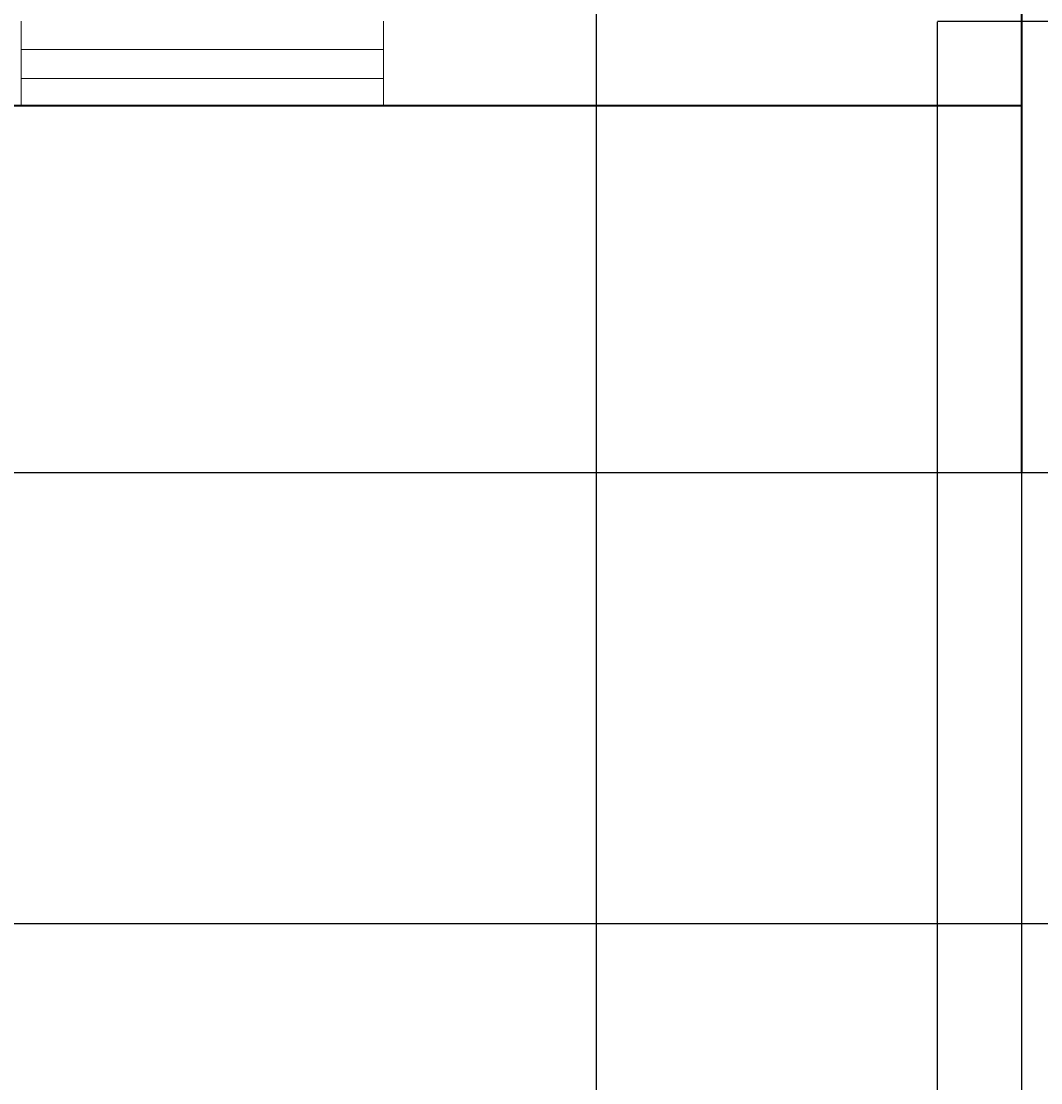
# Model space of a CAD drawing. Units: inches. Extents: x 867 to 1667, y -234 to 788.
# Tile 21 of 42: x 1462 to 1571, y -121 to -8. Entities that reach past the tile are written whole.
import ezdxf

# ---------------------------------------------------------------- set-up
doc = ezdxf.new("R2010")
doc.units = ezdxf.units.IN
doc.header["$MEASUREMENT"] = 0
for name, color, linetype, lineweight in [('A-ANNO-DIMS', 2, 'Continuous', 18), ('A-FLOR-OTLN', 7, 'Continuous', 25), ('A-Glaz', 92, 'Continuous', 18), ('A-Wall', 7, 'Continuous', 35)]:
    doc.layers.add(name, color=color, linetype=linetype, lineweight=lineweight)
doc.styles.get("Standard").update_dxf_attribs({"font": 'arial.ttf'})
doc.dimstyles.get("Standard").update_dxf_attribs({"dimtxt": 0.6875, "dimasz": 0.18, "dimexe": 0.18, "dimexo": 0.0625, "dimgap": 0.09, "dimtad": 0, "dimdec": 4, "dimzin": 0, "dimdsep": 46, "dimlunit": 4, "dimtxsty": 'Standard', "dimcen": 0.09, "dimadec": 0, "dimazin": 0, "dimtfac": 1, "dimtdec": 4, "dimtofl": 0, "dimtmove": 0, "dimatfit": 3, "dimfxl": 1, "dimtolj": 1, "dimtzin": 0, "dimarcsym": 0})

# ---------------------------------------------------------------- blocks, each defined once
blk = doc.blocks.new('WIN-38_58IN')
for p, q in [((0, 9), (0, 0)), ((38.58, 0), (38.58, 9)), ((0, 6), (38.58, 6)), ((0, 2.92), (38.58, 2.92)), ((0, 0), (38.58, 0))]:
    blk.add_line(p, q)
blk = doc.blocks.new('*D27')
at = {"layer": 'A-ANNO-DIMS', "color": 0, "lineweight": -2, "transparency": 16777216}
for p, q in [((1070.89, -55.97), (1070.89, -233.54)), ((1525.26, -186.47), (1525.26, -233.54)), ((1071.07, -233.36), (1296.81, -233.36)), ((1525.08, -233.36), (1299.34, -233.36))]:
    blk.add_line(p, q, dxfattribs=at)
at = {"layer": 'A-ANNO-DIMS', "color": 0, "transparency": 16777216}
for points in [[(1071.07, -233.33), (1071.07, -233.39), (1070.89, -233.36)], [(1525.08, -233.33), (1525.08, -233.39), (1525.26, -233.36)]]:
    blk.add_solid(points, dxfattribs=at)
at = {"layer": 'Defpoints', "color": 0, "transparency": 16777216}
for p in [(1070.89, -55.91), (1525.26, -186.41), (1525.26, -233.36)]:
    blk.add_point(p, dxfattribs=at)
at = {"layer": 'A-ANNO-DIMS', "color": 0, "transparency": 16777216, "insert": (1298.08, -233.36), "char_height": 0.688, "attachment_point": 5}
blk.add_mtext('\\A1;454.4', dxfattribs=at)
blk = doc.blocks.new('*D38')
at = {"layer": 'A-ANNO-DIMS', "color": 0, "lineweight": -2, "transparency": 16777216}
for p, q in [((1403.89, -7.95), (1403.89, -233.54)), ((1559.89, -7.95), (1559.89, -233.54)), ((1404.07, -233.36), (1481.07, -233.36)), ((1559.71, -233.36), (1482.7, -233.36))]:
    blk.add_line(p, q, dxfattribs=at)
at = {"layer": 'A-ANNO-DIMS', "color": 0, "transparency": 16777216}
for points in [[(1404.07, -233.33), (1404.07, -233.39), (1403.89, -233.36)], [(1559.71, -233.33), (1559.71, -233.39), (1559.89, -233.36)]]:
    blk.add_solid(points, dxfattribs=at)
at = {"layer": 'Defpoints', "color": 0, "transparency": 16777216}
for p in [(1403.89, -7.88), (1559.89, -7.88), (1559.89, -233.36)]:
    blk.add_point(p, dxfattribs=at)
at = {"layer": 'A-ANNO-DIMS', "color": 0, "transparency": 16777216, "insert": (1481.89, -233.36), "char_height": 0.688, "attachment_point": 5}
blk.add_mtext('\\A1;156', dxfattribs=at)
blk = doc.blocks.new('*D51')
at = {"layer": 'A-ANNO-DIMS', "color": 0, "lineweight": -2, "transparency": 16777216}
for p, q in [((1391.95, -55.91), (1667.02, -55.91)), ((1666.84, -56.09), (1666.84, -79.31)), ((1666.84, -103.73), (1666.84, -80.51)), ((1391.95, -103.91), (1667.02, -103.91))]:
    blk.add_line(p, q, dxfattribs=at)
at = {"layer": 'A-ANNO-DIMS', "color": 0, "transparency": 16777216}
for points in [[(1666.81, -56.09), (1666.87, -56.09), (1666.84, -55.91)], [(1666.81, -103.73), (1666.87, -103.73), (1666.84, -103.91)]]:
    blk.add_solid(points, dxfattribs=at)
at = {"layer": 'Defpoints', "color": 0, "transparency": 16777216}
for p in [(1391.89, -55.91), (1391.89, -103.91), (1666.84, -103.91)]:
    blk.add_point(p, dxfattribs=at)
at = {"layer": 'A-ANNO-DIMS', "color": 0, "transparency": 16777216, "insert": (1666.84, -79.91), "char_height": 0.688, "attachment_point": 5, "rotation": 90}
blk.add_mtext('\\A1;48', dxfattribs=at)
blk = doc.blocks.new('*D55')
at = {"layer": 'A-ANNO-DIMS', "color": 0, "lineweight": -2, "transparency": 16777216}
for p, q in [((1523.6, 257.55), (1523.6, -233.54)), ((1568.89, 257.55), (1568.89, -233.54)), ((1523.78, -233.36), (1544.71, -233.36)), ((1568.71, -233.36), (1547.78, -233.36))]:
    blk.add_line(p, q, dxfattribs=at)
at = {"layer": 'A-ANNO-DIMS', "color": 0, "transparency": 16777216}
for points in [[(1523.78, -233.33), (1523.78, -233.39), (1523.6, -233.36)], [(1568.71, -233.33), (1568.71, -233.39), (1568.89, -233.36)]]:
    blk.add_solid(points, dxfattribs=at)
at = {"layer": 'Defpoints', "color": 0, "transparency": 16777216}
for p in [(1523.6, 257.62), (1568.89, 257.62), (1568.89, -233.36)]:
    blk.add_point(p, dxfattribs=at)
at = {"layer": 'A-ANNO-DIMS', "color": 0, "transparency": 16777216, "insert": (1546.24, -233.36), "char_height": 0.688, "attachment_point": 5}
blk.add_mtext('\\A1;45.285', dxfattribs=at)
blk = doc.blocks.new('*D59')
at = {"layer": 'A-ANNO-DIMS', "color": 0, "lineweight": -2, "transparency": 16777216}
for p, q in [((1559.95, 24.65), (1667.02, 24.65)), ((1666.84, 24.47), (1666.84, 9.9)), ((1666.84, -7.7), (1666.84, 6.87)), ((1559.95, -7.88), (1667.02, -7.88))]:
    blk.add_line(p, q, dxfattribs=at)
at = {"layer": 'A-ANNO-DIMS', "color": 0, "transparency": 16777216}
for points in [[(1666.81, 24.47), (1666.87, 24.47), (1666.84, 24.65)], [(1666.81, -7.7), (1666.87, -7.7), (1666.84, -7.88)]]:
    blk.add_solid(points, dxfattribs=at)
at = {"layer": 'Defpoints', "color": 0, "transparency": 16777216}
for p in [(1559.89, 24.65), (1666.84, 24.65), (1559.89, -7.88)]:
    blk.add_point(p, dxfattribs=at)
at = {"layer": 'A-ANNO-DIMS', "color": 0, "transparency": 16777216, "insert": (1666.84, 8.38), "char_height": 0.688, "attachment_point": 5, "rotation": 90}
blk.add_mtext('\\A1;32.534', dxfattribs=at)

msp = doc.modelspace()

# ---------------------------------------------------------------- linework, layer by layer
at = {"layer": 'A-FLOR-OTLN'}
msp.add_line((1355.8866, -55.9081), (1568.8866, -55.9081), dxfattribs=at)
at = {"layer": 'A-Wall'}
for p, q in [((1568.8866, 145.117), (1568.8866, -55.9081)), ((1568.8866, -16.883), (1355.8866, -16.883))]:
    msp.add_line(p, q, dxfattribs=at)

# ---------------------------------------------------------------- block references
at = {"layer": 'A-Glaz'}
msp.add_blockref('WIN-38_58IN', (1462.3871, -16.883), dxfattribs=at)

# ---------------------------------------------------------------- dimensions: what is measured, and where the dimension line sits
at = {"layer": 'A-ANNO-DIMS'}
for base, p1, p2, override, picture, middle in [((1568.8866, -233.3581), (1523.6015, 257.617), (1568.8866, 257.617), {"dimdec": 3, "dimlfac": 1, "dimrnd": 0, "dimzin": 0, "dimdsep": 46, "dimlunit": 2}, '*D55', (1546.2441, -233.3581)), ((1559.8866, -233.3581), (1403.8866, -7.883), (1559.8866, -7.883), {"dimdec": 0, "dimlfac": 1, "dimrnd": 0, "dimzin": 0, "dimdsep": 46, "dimlunit": 2}, '*D38', (1481.8866, -233.3581)), ((1525.2648, -233.3581), (1070.8866, -55.9081), (1525.2648, -186.4081), {"dimdec": 1, "dimlfac": 1, "dimrnd": 0, "dimzin": 0, "dimdsep": 46, "dimlunit": 2}, '*D27', (1298.0757, -233.3581))]:
    dim = msp.add_linear_dim(base=base, p1=p1, p2=p2, dimstyle='Standard', override=override, dxfattribs=at)
    dim.commit()
    dim.dimension.update_dxf_attribs({"geometry": picture, "text_midpoint": middle})
for base, p1, p2, override, picture, middle in [((1666.8366, 24.6511), (1559.8866, -7.883), (1559.8866, 24.6511), {"dimdec": 3, "dimlfac": 1, "dimrnd": 0, "dimzin": 0, "dimdsep": 46, "dimlunit": 2}, '*D59', (1666.8366, 8.3841)), ((1666.8366, -103.9081), (1391.8866, -55.9081), (1391.8866, -103.9081), {"dimdec": 0, "dimlfac": 1, "dimrnd": 0, "dimzin": 0, "dimdsep": 46, "dimlunit": 2}, '*D51', (1666.8366, -79.9081))]:
    dim = msp.add_linear_dim(base=base, p1=p1, p2=p2, angle=90, dimstyle='Standard', override=override, dxfattribs=at)
    dim.commit()
    dim.dimension.update_dxf_attribs({"geometry": picture, "text_midpoint": middle})

doc.saveas('drawing.dxf')
